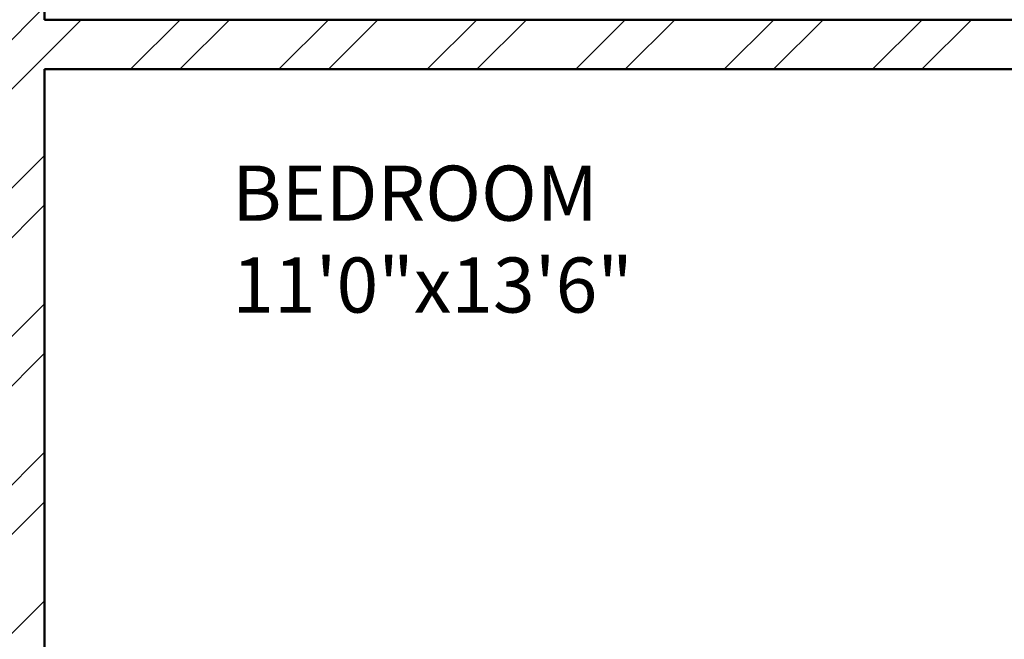
# Model space of a CAD drawing. Units: inches. Extents: x 963 to 2075, y 289 to 2657.
# Tile 43 of 98: x 1511 to 1600, y 1658 to 1714. Entities that reach past the tile are written whole.
import ezdxf

# ---------------------------------------------------------------- set-up
doc = ezdxf.new("R2010")
doc.units = ezdxf.units.IN
for name, color, linetype, lineweight in [('A-AREA-IDEN', 7, 'Continuous', 18), ('A-WALL', 7, 'Continuous', 50), ('A-WALL-PATT', 8, 'Continuous', 13)]:
    doc.layers.add(name, color=color, linetype=linetype, lineweight=lineweight)
doc.styles.get("Standard").update_dxf_attribs({"font": 'arial.ttf'})

msp = doc.modelspace()

# ---------------------------------------------------------------- hatches: boundary and pattern name
at = {"layer": 'A-WALL-PATT'}
h = msp.add_hatch(dxfattribs=at)
h.set_pattern_fill('ANSI32', color=256)
h.paths.add_polyline_path([(1296.922, 2558.318), (1203.922, 2558.318), (1203.922, 2493.818), (1191.533, 2493.818), (1191.533, 2489.318), (1211.063, 2489.318), (1211.063, 2492.02), (1211.063, 2493.818), (1208.422, 2493.818), (1208.422, 2553.818), (1292.422, 2553.818), (1292.422, 2538.863), (1296.922, 2538.863)])
h.paths.add_polyline_path([(1442.422, 2558.318), (1349.422, 2558.318), (1349.422, 2538.943), (1353.922, 2538.943), (1353.922, 2553.818), (1437.922, 2553.818), (1437.922, 2493.818), (1434.542, 2493.818), (1434.542, 2489.318), (1448.311, 2489.318), (1448.311, 2491.568), (1448.311, 2493.818), (1442.422, 2493.818)])
h.paths.add_polyline_path([(1415.554, 2491.568), (1415.554, 2493.818), (1340.941, 2493.818), (1340.941, 2489.318), (1371.922, 2489.318), (1371.922, 2378.318), (1367.596, 2378.318), (1367.596, 2373.818), (1371.922, 2373.818), (1371.922, 2355.185), (1376.422, 2355.185), (1376.422, 2489.318), (1415.554, 2489.318)])
h.paths.add_polyline_path([(1304.941, 2491.568), (1304.941, 2493.818), (1296.922, 2493.818), (1296.922, 2514.863), (1292.422, 2514.863), (1292.422, 2493.818), (1232.808, 2493.818), (1232.808, 2489.318), (1256.422, 2489.318), (1256.422, 2327.318), (1253.714, 2327.318), (1253.714, 2322.818), (1328.422, 2322.818), (1328.422, 2331.147), (1323.922, 2331.147), (1323.922, 2327.318), (1260.922, 2327.318), (1260.922, 2373.818), (1323.922, 2373.818), (1323.922, 2357.812), (1328.422, 2357.812), (1328.422, 2373.818), (1346.007, 2373.818), (1346.007, 2376.068), (1346.007, 2378.318), (1260.922, 2378.318), (1260.922, 2489.318), (1304.941, 2489.318)])
h.paths.add_polyline_path([(1226.654, 2327.318), (1124.422, 2327.318), (1124.422, 2347.447), (1119.922, 2347.447), (1119.922, 2322.818), (1163.422, 2322.818), (1163.422, 2305.435), (1165.672, 2305.435), (1167.922, 2305.435), (1167.922, 2322.818), (1226.654, 2322.818), (1226.654, 2325.068)])
h.paths.add_polyline_path([(1095.922, 2489.318), (1124.422, 2489.318), (1131.533, 2489.318), (1131.533, 2491.568), (1131.533, 2493.818), (1119.922, 2493.818), (1091.422, 2493.818), (1091.422, 2417.318), (1095.922, 2417.318), (1119.922, 2417.318), (1119.922, 2407.447), (1124.422, 2407.447), (1124.422, 2421.818), (1095.922, 2421.818)])
h.paths.add_polyline_path([(1512.922, 2558.318), (1508.422, 2558.318), (1508.422, 2493.818), (1503.401, 2493.818), (1503.401, 2489.318), (1508.422, 2489.318), (1508.422, 2327.318), (1376.422, 2327.318), (1376.422, 2330.273), (1371.922, 2330.273), (1371.922, 2298.744), (1376.422, 2298.744), (1376.422, 2322.818), (1508.422, 2322.818), (1508.422, 2165.318), (1504.255, 2165.318), (1504.255, 2160.818), (1508.422, 2160.818), (1508.422, 2108.318), (1512.922, 2108.318), (1512.922, 2160.818), (1516.182, 2160.818), (1516.182, 2163.068), (1516.182, 2165.318), (1512.922, 2165.318), (1512.922, 2322.818), (1644.922, 2322.818), (1644.922, 2298.744), (1649.422, 2298.744), (1649.422, 2322.818), (1649.422, 2330.944), (1647.172, 2330.944), (1644.922, 2330.944), (1644.922, 2327.318), (1512.922, 2327.318), (1512.922, 2489.318), (1516.759, 2489.318), (1516.759, 2491.568), (1516.759, 2493.818), (1512.922, 2493.818)])
h.paths.add_polyline_path([(1671.922, 2558.318), (1578.922, 2558.318), (1578.922, 2493.818), (1573.526, 2493.818), (1573.526, 2489.318), (1586.537, 2489.318), (1586.537, 2491.568), (1586.537, 2493.818), (1583.422, 2493.818), (1583.422, 2553.818), (1667.422, 2553.818), (1667.422, 2541.109), (1671.922, 2541.109)])
h.paths.add_polyline_path([(1681.257, 2493.818), (1671.922, 2493.818), (1671.922, 2517.109), (1667.422, 2517.109), (1667.422, 2493.818), (1610.218, 2493.818), (1610.218, 2489.318), (1644.922, 2489.318), (1644.922, 2357.865), (1649.422, 2357.865), (1649.422, 2373.818), (1652.203, 2373.818), (1652.203, 2375.827), (1652.203, 2378.318), (1649.422, 2378.318), (1649.422, 2489.318), (1681.257, 2489.318), (1681.257, 2491.568)])
h.paths.add_polyline_path([(1821.922, 2558.318), (1728.922, 2558.318), (1728.922, 2541), (1733.422, 2541), (1733.422, 2553.818), (1817.422, 2553.818), (1817.422, 2493.818), (1813.507, 2493.818), (1813.507, 2489.318), (1830.078, 2489.318), (1830.078, 2491.568), (1830.078, 2493.818), (1821.922, 2493.818)])
h.paths.add_polyline_path([(1794.244, 2493.818), (1717.257, 2493.818), (1717.257, 2489.318), (1760.422, 2489.318), (1760.422, 2378.318), (1674.401, 2378.318), (1674.401, 2373.818), (1692.922, 2373.818), (1692.922, 2356.954), (1697.422, 2356.954), (1697.422, 2373.818), (1760.422, 2373.818), (1760.422, 2327.318), (1697.422, 2327.318), (1697.422, 2333.341), (1692.922, 2333.341), (1692.922, 2322.818), (1768.037, 2322.818), (1768.037, 2325.068), (1768.037, 2327.318), (1764.922, 2327.318), (1764.922, 2489.318), (1794.244, 2489.318)])
h.paths.add_polyline_path([(1733.422, 2517), (1728.922, 2517), (1728.922, 2493.818), (1733.422, 2493.818)], flags=17)
h.paths.add_polyline_path([(1929.922, 2493.818), (1890.078, 2493.818), (1890.078, 2489.318), (1896.922, 2489.318), (1925.422, 2489.318), (1925.422, 2421.818), (1896.922, 2421.818), (1896.922, 2408.318), (1901.422, 2408.318), (1901.422, 2417.318), (1925.422, 2417.318), (1929.922, 2417.318)])
h.paths.add_polyline_path([(1901.422, 2348.318), (1896.922, 2348.318), (1896.922, 2327.318), (1800.423, 2327.318), (1800.423, 2322.818), (1853.422, 2322.818), (1853.422, 2309.453), (1857.922, 2309.453), (1857.922, 2322.818), (1901.422, 2322.818)])
h.paths.add_polyline_path([(1857.922, 2249.453), (1853.422, 2249.453), (1853.422, 2214.818), (1686.309, 2214.818), (1686.309, 2210.318), (1853.422, 2210.318), (1853.422, 2202.134), (1857.922, 2202.134), (1857.922, 2210.318)])
h.paths.add_polyline_path([(1857.922, 2142.134), (1853.422, 2142.134), (1853.422, 2115.422), (1841.422, 2115.422), (1841.422, 2088.531), (1841.422, 2046.949), (1845.922, 2046.949), (1845.922, 2110.922), (1905.922, 2110.922), (1905.922, 2092.517), (1910.422, 2092.517), (1910.422, 2115.422), (1857.922, 2115.422)])
h.paths.add_polyline_path([(1532.436, 1482.342), (1573.456, 1482.342), (1573.456, 1501), (1532.436, 1501)], flags=9)
h.paths.add_polyline_path([(1438.658, 1486.302), (1479.678, 1486.302), (1479.678, 1504.96), (1438.658, 1504.96)], flags=9)
h.paths.add_polyline_path([(1411.215, 1365.308), (1659.139, 1365.308), (1659.139, 1402.401), (1411.215, 1402.401)], flags=9)
h.paths.add_polyline_path([(1185.671, 2296.298), (1248.16, 2296.298), (1248.16, 2314.955), (1185.671, 2314.955)], flags=9)
h.paths.add_polyline_path([(1177.31, 2187.35), (1216.15, 2187.35), (1216.15, 2206.007), (1177.31, 2206.007)], flags=9)
h.paths.add_polyline_path([(1295.101, 1602.083), (1328.26, 1602.083), (1328.26, 1620.741), (1295.101, 1620.741)], flags=9)
h.paths.add_polyline_path([(1525.126, 2005.99), (1558.39, 2005.99), (1558.39, 2024.648), (1525.126, 2024.648)], flags=9)
h.paths.add_polyline_path([(1459.606, 1977.125), (1472.195, 1977.125), (1472.195, 1987.429), (1459.606, 1987.429)], flags=9)
h.paths.add_polyline_path([(1467.815, 2053.676), (1480.018, 2053.676), (1480.018, 2063.979), (1467.815, 2063.979)], flags=9)
h.paths.add_polyline_path([(1555.184, 2119.02), (1584.563, 2119.02), (1584.563, 2137.678), (1555.184, 2137.678)], flags=25)
h.paths.add_polyline_path([(1405.389, 2115.291), (1444.478, 2115.291), (1444.478, 2133.948), (1405.389, 2133.948)], flags=25)
h.paths.add_polyline_path([(1698.482, 2004.259), (1727.695, 2004.259), (1727.695, 2022.916), (1698.482, 2022.916)], flags=9)
h.paths.add_polyline_path([(1612.158, 1972.855), (1629.016, 1972.855), (1629.016, 1983.159), (1612.158, 1983.159)], flags=9)
h.paths.add_polyline_path([(1608.289, 2060.036), (1625.147, 2060.036), (1625.147, 2070.34), (1608.289, 2070.34)], flags=9)
h.paths.add_polyline_path([(1527.954, 1684.402), (1566.795, 1684.402), (1566.795, 1703.06), (1527.954, 1703.06)], flags=9)
h.paths.add_polyline_path([(1422.792, 1683.59), (1461.633, 1683.59), (1461.633, 1702.247), (1422.792, 1702.247)], flags=9)
h.paths.add_polyline_path([(1531.262, 1732.459), (1574.015, 1732.459), (1574.015, 1751.116), (1531.262, 1751.116)], flags=9)
h.paths.add_polyline_path([(1402.872, 1732.845), (1439.799, 1732.845), (1439.799, 1751.502), (1402.872, 1751.502)], flags=9)
h.paths.add_polyline_path([(1243.122, 1923.132), (1281.962, 1923.132), (1281.962, 1941.79), (1243.122, 1941.79)], flags=9)
h.paths.add_polyline_path([(1181.752, 1792.268), (1244.241, 1792.268), (1244.241, 1810.926), (1181.752, 1810.926)], flags=9)
h.paths.add_polyline_path([(1265.822, 1670.3), (1316.071, 1670.3), (1316.071, 1688.957), (1265.822, 1688.957)], flags=9)
h.paths.add_polyline_path([(1140.263, 1676.054), (1179.104, 1676.054), (1179.104, 1694.711), (1140.263, 1694.711)], flags=9)
h.paths.add_polyline_path([(1107.49, 1490.889), (1143.374, 1490.889), (1143.374, 1509.546), (1107.49, 1509.546)], flags=9)
h.paths.add_polyline_path([(1217.584, 1483.899), (1246.741, 1483.899), (1246.741, 1502.556), (1217.584, 1502.556)], flags=9)
h.paths.add_polyline_path([(1389.21, 1486.919), (1418.367, 1486.919), (1418.367, 1505.576), (1389.21, 1505.576)], flags=9)
h.paths.add_polyline_path([(1672.208, 1602.083), (1705.366, 1602.083), (1705.366, 1620.741), (1672.208, 1620.741)], flags=9)
h.paths.add_polyline_path([(1752.082, 1522.638), (1781.24, 1522.638), (1781.24, 1541.295), (1752.082, 1541.295)], flags=9)
h.paths.add_polyline_path([(1848.275, 1491.26), (1884.158, 1491.26), (1884.158, 1509.918), (1848.275, 1509.918)], flags=9)
h.paths.add_polyline_path([(1822.47, 1685.62), (1861.31, 1685.62), (1861.31, 1704.278), (1822.47, 1704.278)], flags=9)
h.paths.add_polyline_path([(1713.195, 1672.232), (1763.444, 1672.232), (1763.444, 1690.889), (1713.195, 1690.889)], flags=9)
h.paths.add_polyline_path([(1736.619, 1790.578), (1799.109, 1790.578), (1799.109, 1809.235), (1736.619, 1809.235)], flags=9)
h.paths.add_polyline_path([(1691.491, 1916.355), (1730.332, 1916.355), (1730.332, 1935.013), (1691.491, 1935.013)], flags=9)
h.paths.add_polyline_path([(1764.872, 1973.922), (1794.306, 1973.922), (1794.306, 1992.58), (1764.872, 1992.58)], flags=9)
h.paths.add_polyline_path([(1767.854, 2034.017), (1797.288, 2034.017), (1797.288, 2052.674), (1767.854, 2052.674)], flags=9)
h.paths.add_polyline_path([(1851.593, 2060.331), (1880.751, 2060.331), (1880.751, 2078.989), (1851.593, 2078.989)], flags=25)
h.paths.add_polyline_path([(1688.491, 2086.874), (1727.332, 2086.874), (1727.332, 2105.531), (1688.491, 2105.531)], flags=9)
h.paths.add_polyline_path([(1537.743, 2293.581), (1580.495, 2293.581), (1580.495, 2312.239), (1537.743, 2312.239)], flags=25)
h.paths.add_polyline_path([(1425.587, 2296.109), (1468.34, 2296.109), (1468.34, 2314.766), (1425.587, 2314.766)], flags=25)
h.paths.add_polyline_path([(1278.518, 2004.184), (1307.72, 2004.184), (1307.72, 2022.841), (1278.518, 2022.841)], flags=9)
h.paths.add_polyline_path([(1193.282, 1973.635), (1222.715, 1973.635), (1222.715, 1992.292), (1193.282, 1992.292)], flags=9)
h.paths.add_polyline_path([(1192.411, 2040.577), (1221.845, 2040.577), (1221.845, 2059.234), (1192.411, 2059.234)], flags=9)
h.paths.add_polyline_path([(1130.603, 1951.393), (1159.76, 1951.393), (1159.76, 1970.05), (1130.603, 1970.05)], flags=9)
h.paths.add_polyline_path([(1132.827, 2052.494), (1161.984, 2052.494), (1161.984, 2071.151), (1132.827, 2071.151)], flags=9)
h.paths.add_polyline_path([(1265.128, 2334.619), (1315.377, 2334.619), (1315.377, 2353.277), (1265.128, 2353.277)], flags=25)
h.paths.add_polyline_path([(1136.741, 2330.785), (1175.582, 2330.785), (1175.582, 2349.443), (1136.741, 2349.443)], flags=9)
h.paths.add_polyline_path([(1287.422, 2417.204), (1320.58, 2417.204), (1320.58, 2435.861), (1287.422, 2435.861)], flags=25)
h.paths.add_polyline_path([(1430.988, 2329.159), (1469.828, 2329.159), (1469.828, 2347.816), (1430.988, 2347.816)], flags=25)
h.paths.add_polyline_path([(1525.424, 2329.213), (1564.264, 2329.213), (1564.264, 2347.87), (1525.424, 2347.87)], flags=25)
h.paths.add_polyline_path([(1684.525, 2382.799), (1717.683, 2382.799), (1717.683, 2401.457), (1684.525, 2401.457)], flags=25)
h.paths.add_polyline_path([(1704.805, 2340.293), (1755.054, 2340.293), (1755.054, 2358.95), (1704.805, 2358.95)], flags=25)
h.paths.add_polyline_path([(1694.113, 2287.757), (1756.602, 2287.757), (1756.602, 2306.414), (1694.113, 2306.414)], flags=9)
h.paths.add_polyline_path([(1815.778, 2329.861), (1854.618, 2329.861), (1854.618, 2348.518), (1815.778, 2348.518)], flags=9)
h.paths.add_polyline_path([(1842.873, 2514.256), (1878.756, 2514.256), (1878.756, 2532.914), (1842.873, 2532.914)], flags=9)
h.paths.add_polyline_path([(1769.513, 2531.447), (1798.671, 2531.447), (1798.671, 2550.104), (1769.513, 2550.104)], flags=25)
h.paths.add_polyline_path([(1594.772, 2518.468), (1623.93, 2518.468), (1623.93, 2537.125), (1594.772, 2537.125)], flags=25)
h.paths.add_polyline_path([(1520.723, 2516.185), (1556.606, 2516.185), (1556.606, 2534.842), (1520.723, 2534.842)], flags=25)
h.paths.add_polyline_path([(1464.456, 2516.694), (1500.34, 2516.694), (1500.34, 2535.351), (1464.456, 2535.351)], flags=25)
h.paths.add_polyline_path([(1365.696, 2528.97), (1394.854, 2528.97), (1394.854, 2547.627), (1365.696, 2547.627)], flags=25)
h.paths.add_polyline_path([(1222.838, 2516.231), (1251.995, 2516.231), (1251.995, 2534.889), (1222.838, 2534.889)], flags=25)
h.paths.add_polyline_path([(1104.545, 2509.6), (1140.429, 2509.6), (1140.429, 2528.257), (1104.545, 2528.257)], flags=9)
h = msp.add_hatch(dxfattribs=at)
h.set_pattern_fill('ANSI32', color=256)
h.paths.add_polyline_path([(1335.968, 2212.568), (1335.968, 2214.818), (1167.922, 2214.818), (1167.922, 2245.435), (1163.422, 2245.435), (1163.422, 2210.318), (1163.422, 2194.812), (1167.922, 2194.812), (1167.922, 2210.318), (1335.968, 2210.318)])
h.paths.add_polyline_path([(1532.436, 1482.342), (1573.456, 1482.342), (1573.456, 1501), (1532.436, 1501)], flags=9)
h.paths.add_polyline_path([(1438.658, 1486.302), (1479.678, 1486.302), (1479.678, 1504.96), (1438.658, 1504.96)], flags=9)
h.paths.add_polyline_path([(1411.215, 1365.308), (1659.139, 1365.308), (1659.139, 1402.401), (1411.215, 1402.401)], flags=9)
h.paths.add_polyline_path([(1185.671, 2296.298), (1248.16, 2296.298), (1248.16, 2314.955), (1185.671, 2314.955)], flags=9)
h.paths.add_polyline_path([(1177.31, 2187.35), (1216.15, 2187.35), (1216.15, 2206.007), (1177.31, 2206.007)], flags=9)
h.paths.add_polyline_path([(1295.101, 1602.083), (1328.26, 1602.083), (1328.26, 1620.741), (1295.101, 1620.741)], flags=9)
h.paths.add_polyline_path([(1525.126, 2005.99), (1558.39, 2005.99), (1558.39, 2024.648), (1525.126, 2024.648)], flags=9)
h.paths.add_polyline_path([(1459.606, 1977.125), (1472.195, 1977.125), (1472.195, 1987.429), (1459.606, 1987.429)], flags=9)
h.paths.add_polyline_path([(1467.815, 2053.676), (1480.018, 2053.676), (1480.018, 2063.979), (1467.815, 2063.979)], flags=9)
h.paths.add_polyline_path([(1555.184, 2119.02), (1584.563, 2119.02), (1584.563, 2137.678), (1555.184, 2137.678)], flags=9)
h.paths.add_polyline_path([(1405.389, 2115.291), (1444.478, 2115.291), (1444.478, 2133.948), (1405.389, 2133.948)], flags=9)
h.paths.add_polyline_path([(1698.482, 2004.259), (1727.695, 2004.259), (1727.695, 2022.916), (1698.482, 2022.916)], flags=9)
h.paths.add_polyline_path([(1612.158, 1972.855), (1629.016, 1972.855), (1629.016, 1983.159), (1612.158, 1983.159)], flags=9)
h.paths.add_polyline_path([(1608.289, 2060.036), (1625.147, 2060.036), (1625.147, 2070.34), (1608.289, 2070.34)], flags=9)
h.paths.add_polyline_path([(1527.954, 1684.402), (1566.795, 1684.402), (1566.795, 1703.06), (1527.954, 1703.06)], flags=9)
h.paths.add_polyline_path([(1422.792, 1683.59), (1461.633, 1683.59), (1461.633, 1702.247), (1422.792, 1702.247)], flags=9)
h.paths.add_polyline_path([(1531.262, 1732.459), (1574.015, 1732.459), (1574.015, 1751.116), (1531.262, 1751.116)], flags=9)
h.paths.add_polyline_path([(1402.872, 1732.845), (1439.799, 1732.845), (1439.799, 1751.502), (1402.872, 1751.502)], flags=9)
h.paths.add_polyline_path([(1243.122, 1923.132), (1281.962, 1923.132), (1281.962, 1941.79), (1243.122, 1941.79)], flags=9)
h.paths.add_polyline_path([(1181.752, 1792.268), (1244.241, 1792.268), (1244.241, 1810.926), (1181.752, 1810.926)], flags=9)
h.paths.add_polyline_path([(1265.822, 1670.3), (1316.071, 1670.3), (1316.071, 1688.957), (1265.822, 1688.957)], flags=9)
h.paths.add_polyline_path([(1140.263, 1676.054), (1179.104, 1676.054), (1179.104, 1694.711), (1140.263, 1694.711)], flags=9)
h.paths.add_polyline_path([(1107.49, 1490.889), (1143.374, 1490.889), (1143.374, 1509.546), (1107.49, 1509.546)], flags=9)
h.paths.add_polyline_path([(1217.584, 1483.899), (1246.741, 1483.899), (1246.741, 1502.556), (1217.584, 1502.556)], flags=9)
h.paths.add_polyline_path([(1389.21, 1486.919), (1418.367, 1486.919), (1418.367, 1505.576), (1389.21, 1505.576)], flags=9)
h.paths.add_polyline_path([(1672.208, 1602.083), (1705.366, 1602.083), (1705.366, 1620.741), (1672.208, 1620.741)], flags=9)
h.paths.add_polyline_path([(1752.082, 1522.638), (1781.24, 1522.638), (1781.24, 1541.295), (1752.082, 1541.295)], flags=9)
h.paths.add_polyline_path([(1848.275, 1491.26), (1884.158, 1491.26), (1884.158, 1509.918), (1848.275, 1509.918)], flags=9)
h.paths.add_polyline_path([(1822.47, 1685.62), (1861.31, 1685.62), (1861.31, 1704.278), (1822.47, 1704.278)], flags=9)
h.paths.add_polyline_path([(1713.195, 1672.232), (1763.444, 1672.232), (1763.444, 1690.889), (1713.195, 1690.889)], flags=9)
h.paths.add_polyline_path([(1736.619, 1790.578), (1799.109, 1790.578), (1799.109, 1809.235), (1736.619, 1809.235)], flags=9)
h.paths.add_polyline_path([(1691.491, 1916.355), (1730.332, 1916.355), (1730.332, 1935.013), (1691.491, 1935.013)], flags=9)
h.paths.add_polyline_path([(1764.872, 1973.922), (1794.306, 1973.922), (1794.306, 1992.58), (1764.872, 1992.58)], flags=9)
h.paths.add_polyline_path([(1767.854, 2034.017), (1797.288, 2034.017), (1797.288, 2052.674), (1767.854, 2052.674)], flags=9)
h.paths.add_polyline_path([(1851.593, 2060.331), (1880.751, 2060.331), (1880.751, 2078.989), (1851.593, 2078.989)], flags=9)
h.paths.add_polyline_path([(1688.491, 2086.874), (1727.332, 2086.874), (1727.332, 2105.531), (1688.491, 2105.531)], flags=9)
h.paths.add_polyline_path([(1537.743, 2293.581), (1580.495, 2293.581), (1580.495, 2312.239), (1537.743, 2312.239)], flags=9)
h.paths.add_polyline_path([(1425.587, 2296.109), (1468.34, 2296.109), (1468.34, 2314.766), (1425.587, 2314.766)], flags=9)
h.paths.add_polyline_path([(1278.518, 2004.184), (1307.72, 2004.184), (1307.72, 2022.841), (1278.518, 2022.841)], flags=9)
h.paths.add_polyline_path([(1193.282, 1973.635), (1222.715, 1973.635), (1222.715, 1992.292), (1193.282, 1992.292)], flags=9)
h.paths.add_polyline_path([(1192.411, 2040.577), (1221.845, 2040.577), (1221.845, 2059.234), (1192.411, 2059.234)], flags=9)
h.paths.add_polyline_path([(1130.603, 1951.393), (1159.76, 1951.393), (1159.76, 1970.05), (1130.603, 1970.05)], flags=9)
h.paths.add_polyline_path([(1132.827, 2052.494), (1161.984, 2052.494), (1161.984, 2071.151), (1132.827, 2071.151)], flags=9)
h.paths.add_polyline_path([(1265.128, 2334.619), (1315.377, 2334.619), (1315.377, 2353.277), (1265.128, 2353.277)], flags=9)
h.paths.add_polyline_path([(1136.741, 2330.785), (1175.582, 2330.785), (1175.582, 2349.443), (1136.741, 2349.443)], flags=9)
h.paths.add_polyline_path([(1287.422, 2417.204), (1320.58, 2417.204), (1320.58, 2435.861), (1287.422, 2435.861)], flags=9)
h.paths.add_polyline_path([(1430.988, 2329.159), (1469.828, 2329.159), (1469.828, 2347.816), (1430.988, 2347.816)], flags=9)
h.paths.add_polyline_path([(1525.424, 2329.213), (1564.264, 2329.213), (1564.264, 2347.87), (1525.424, 2347.87)], flags=9)
h.paths.add_polyline_path([(1684.525, 2382.799), (1717.683, 2382.799), (1717.683, 2401.457), (1684.525, 2401.457)], flags=9)
h.paths.add_polyline_path([(1704.805, 2340.293), (1755.054, 2340.293), (1755.054, 2358.95), (1704.805, 2358.95)], flags=9)
h.paths.add_polyline_path([(1694.113, 2287.757), (1756.602, 2287.757), (1756.602, 2306.414), (1694.113, 2306.414)], flags=9)
h.paths.add_polyline_path([(1815.778, 2329.861), (1854.618, 2329.861), (1854.618, 2348.518), (1815.778, 2348.518)], flags=9)
h.paths.add_polyline_path([(1842.873, 2514.256), (1878.756, 2514.256), (1878.756, 2532.914), (1842.873, 2532.914)], flags=9)
h.paths.add_polyline_path([(1769.513, 2531.447), (1798.671, 2531.447), (1798.671, 2550.104), (1769.513, 2550.104)], flags=9)
h.paths.add_polyline_path([(1594.772, 2518.468), (1623.93, 2518.468), (1623.93, 2537.125), (1594.772, 2537.125)], flags=9)
h.paths.add_polyline_path([(1520.723, 2516.185), (1556.606, 2516.185), (1556.606, 2534.842), (1520.723, 2534.842)], flags=9)
h.paths.add_polyline_path([(1464.456, 2516.694), (1500.34, 2516.694), (1500.34, 2535.351), (1464.456, 2535.351)], flags=9)
h.paths.add_polyline_path([(1365.696, 2528.97), (1394.854, 2528.97), (1394.854, 2547.627), (1365.696, 2547.627)], flags=9)
h.paths.add_polyline_path([(1222.838, 2516.231), (1251.995, 2516.231), (1251.995, 2534.889), (1222.838, 2534.889)], flags=9)
h.paths.add_polyline_path([(1104.545, 2509.6), (1140.429, 2509.6), (1140.429, 2528.257), (1104.545, 2528.257)], flags=9)
h = msp.add_hatch(dxfattribs=at)
h.set_pattern_fill('ANSI32', color=256)
h.paths.add_polyline_path([(1473.609, 2163.068), (1473.609, 2165.318), (1376.422, 2165.318), (1376.422, 2227.983), (1371.922, 2227.983), (1371.922, 2214.818), (1368.405, 2214.818), (1368.405, 2210.318), (1371.922, 2210.318), (1371.922, 2160.818), (1395.922, 2160.818), (1395.922, 2090.318), (1217.345, 2090.318), (1217.345, 2085.818), (1395.922, 2085.818), (1458.922, 2085.818), (1458.922, 2108.318), (1454.422, 2108.318), (1454.422, 2090.318), (1400.422, 2090.318), (1400.422, 2160.818), (1473.609, 2160.818)])
h.paths.add_polyline_path([(1649.422, 2210.318), (1653.225, 2210.318), (1653.225, 2214.818), (1649.422, 2214.818), (1649.422, 2227.983), (1644.922, 2227.983), (1644.922, 2165.318), (1550.099, 2165.318), (1550.099, 2160.818), (1620.922, 2160.818), (1620.922, 2112.818), (1555.446, 2112.818), (1555.446, 2108.318), (1584.327, 2108.318), (1584.327, 2084.916), (1588.827, 2084.916), (1588.827, 2108.318), (1625.422, 2108.318), (1667.951, 2108.318), (1667.951, 2022.667), (1588.827, 2022.667), (1588.827, 2047.408), (1584.327, 2047.408), (1584.327, 1996.003), (1588.827, 1996.003), (1588.827, 2018.318), (1667.951, 2018.167), (1667.951, 1928.318), (1625.422, 1928.318), (1625.422, 1923.818), (1672.451, 1923.818), (1672.451, 1928.318), (1672.451, 1946.663), (1785.446, 1946.663), (1785.446, 1951.163), (1743.034, 1951.163), (1743.034, 2017.922), (1841.422, 2017.922), (1841.422, 2014.775), (1845.922, 2014.775), (1845.922, 2017.922), (1905.922, 2017.922), (1905.922, 1987.511), (1910.422, 1987.511), (1910.422, 2022.422), (1910.422, 2068.517), (1905.922, 2068.517), (1905.922, 2022.422), (1845.922, 2022.422), (1845.922, 2025.851), (1843.672, 2025.851), (1841.422, 2025.851), (1841.422, 2022.422), (1743.034, 2022.422), (1743.034, 2084.031), (1768.451, 2084.031), (1785.446, 2084.031), (1785.446, 2088.531), (1672.451, 2088.531), (1672.451, 2112.818), (1667.951, 2112.818), (1625.422, 2112.818), (1625.422, 2160.818), (1649.422, 2160.818)])
h.paths.add_polyline_path([(1672.451, 2084.031), (1738.534, 2084.031), (1738.534, 1951.163), (1672.451, 1951.163)], flags=16)
h.paths.add_polyline_path([(1672.451, 2084.031), (1738.534, 2084.031), (1705.492, 2017.597)], flags=0)
h.paths.add_polyline_path([(1262.766, 2085.818), (1258.266, 2085.818), (1258.266, 2023.278), (1184.422, 2023.278), (1184.422, 2018.778), (1258.266, 2018.778), (1258.266, 1950.818), (1262.766, 1950.818)])
h.paths.add_polyline_path([(1312.266, 2085.818), (1307.766, 2085.818), (1307.766, 1950.818), (1312.266, 1950.818)])
h.paths.add_polyline_path([(1458.922, 1950.818), (1395.922, 1950.818), (1216.568, 1950.818), (1216.568, 1946.318), (1346.422, 1946.318), (1395.922, 1946.318), (1395.922, 1875.818), (1371.922, 1875.818), (1371.922, 1826.318), (1368.931, 1826.318), (1368.931, 1821.818), (1371.922, 1821.818), (1371.922, 1813.622), (1376.422, 1813.622), (1376.422, 1871.318), (1474.504, 1871.318), (1474.504, 1873.568), (1474.504, 1875.818), (1400.422, 1875.818), (1400.422, 1946.318), (1454.422, 1946.318), (1454.422, 1928.318), (1458.922, 1928.318)])
h.paths.add_polyline_path([(1184.422, 2120.778), (1167.922, 2120.778), (1167.922, 2134.812), (1165.672, 2134.812), (1163.422, 2134.812), (1163.422, 2120.778), (1119.922, 2120.778), (1119.922, 2098.095), (1124.422, 2098.095), (1124.422, 2116.278), (1167.922, 2116.278), (1179.922, 2116.278), (1179.922, 2045.916), (1184.422, 2045.916), (1184.422, 2090.318), (1184.422, 2116.278)])
h.paths.add_polyline_path([(1124.422, 2018.778), (1179.922, 2018.778), (1179.922, 2016.294), (1184.422, 2016.294), (1184.422, 2023.278), (1184.422, 2026.588), (1182.172, 2026.588), (1179.922, 2026.588), (1179.922, 2023.278), (1124.422, 2023.278), (1124.422, 2074.095), (1119.922, 2074.095), (1119.922, 2018.778), (1119.922, 1979.633), (1124.422, 1979.633)])
h.paths.add_polyline_path([(1184.422, 1925.778), (1184.422, 1946.318), (1184.422, 1996.073), (1182.172, 1996.073), (1179.922, 1996.073), (1179.922, 1925.778), (1124.422, 1925.778), (1124.422, 1955.633), (1119.922, 1955.502), (1119.922, 1921.278), (1158.922, 1921.278), (1158.922, 1909.983), (1163.422, 1909.983), (1163.422, 1921.278), (1184.422, 1921.278)])
h.paths.add_polyline_path([(1341.449, 1826.318), (1163.422, 1826.318), (1163.422, 1849.983), (1158.922, 1849.983), (1158.922, 1821.818), (1158.922, 1804.033), (1163.422, 1804.033), (1163.422, 1821.818), (1341.449, 1821.818)])
h.paths.add_polyline_path([(1222.981, 1713.818), (1163.422, 1713.818), (1163.422, 1744.033), (1161.172, 1744.033), (1158.922, 1744.033), (1158.922, 1713.818), (1119.922, 1713.818), (1119.922, 1694.65), (1124.422, 1694.65), (1124.422, 1709.318), (1158.922, 1709.318), (1222.981, 1709.318)])
h.paths.add_polyline_path([(1328.422, 1713.818), (1252.042, 1713.818), (1252.042, 1711.568), (1252.042, 1709.318), (1256.422, 1709.318), (1256.422, 1547.318), (1232.937, 1547.318), (1232.937, 1545.068), (1232.937, 1542.818), (1292.422, 1542.818), (1292.422, 1527.634), (1296.922, 1527.634), (1296.922, 1542.818), (1299.464, 1542.818), (1299.464, 1547.318), (1260.922, 1547.318), (1260.922, 1658.318), (1343.661, 1658.318), (1343.661, 1660.568), (1343.661, 1662.818), (1328.422, 1662.818), (1328.422, 1676.589), (1327.402, 1676.589), (1323.922, 1676.589), (1323.922, 1662.818), (1260.922, 1662.818), (1260.922, 1709.318), (1323.922, 1709.318), (1323.922, 1699.851), (1328.422, 1699.851)])
h.paths.add_polyline_path([(1649.422, 1875.818), (1625.422, 1875.818), (1625.422, 1928.318), (1620.922, 1928.318), (1588.827, 1928.318), (1588.827, 1950.59), (1584.327, 1950.59), (1584.327, 1928.318), (1555.446, 1928.318), (1555.446, 1923.818), (1620.922, 1923.818), (1620.922, 1875.818), (1548.952, 1875.818), (1548.952, 1873.568), (1548.952, 1871.318), (1644.922, 1871.318), (1644.922, 1813.622), (1649.422, 1813.622), (1649.422, 1821.818), (1652.045, 1821.818), (1652.045, 1824.068), (1652.045, 1826.318), (1649.422, 1826.318)])
h.paths.add_polyline_path([(1512.922, 1871.318), (1516.476, 1871.318), (1516.476, 1875.818), (1512.922, 1875.818), (1512.922, 1923.818), (1512.922, 1928.318), (1512.922, 1930.827), (1508.422, 1930.827), (1508.422, 1875.818), (1504.411, 1875.818), (1504.411, 1871.318), (1508.422, 1871.318), (1508.422, 1713.818), (1376.422, 1713.818), (1376.422, 1743.325), (1371.922, 1743.325), (1371.922, 1709.318), (1371.922, 1706.01), (1376.422, 1706.01), (1376.422, 1709.318), (1508.422, 1709.318), (1508.422, 1547.318), (1501.871, 1547.318), (1501.871, 1542.818), (1508.422, 1542.818), (1508.422, 1482.818), (1508.422, 1436.318), (1512.922, 1436.318), (1512.922, 1542.818), (1519.318, 1542.818), (1519.318, 1545.068), (1519.318, 1547.318), (1512.922, 1547.318), (1512.922, 1709.318), (1644.922, 1709.318), (1644.922, 1707.548), (1649.422, 1707.548), (1649.422, 1709.318), (1649.422, 1743.325), (1644.922, 1743.325), (1644.922, 1713.818), (1512.922, 1713.818)])
h.paths.add_polyline_path([(1129.884, 1545.068), (1129.884, 1547.318), (1124.422, 1547.318), (1095.922, 1547.318), (1095.922, 1614.818), (1124.422, 1614.818), (1124.422, 1619.318), (1095.922, 1619.318), (1091.422, 1619.318), (1091.422, 1542.818), (1095.922, 1542.818), (1119.922, 1542.818), (1129.884, 1542.818)])
h.paths.add_polyline_path([(1208.422, 1542.818), (1211.74, 1542.818), (1211.74, 1547.318), (1198.851, 1547.318), (1198.851, 1542.818), (1203.922, 1542.818), (1203.922, 1478.318), (1208.422, 1478.318), (1296.922, 1478.318), (1296.922, 1503.634), (1292.422, 1503.634), (1292.422, 1482.818), (1208.422, 1482.818)])
h.paths.add_polyline_path([(1430.422, 1542.818), (1435.699, 1542.818), (1435.699, 1545.068), (1435.699, 1547.318), (1422.658, 1547.318), (1422.658, 1545.068), (1422.658, 1542.818), (1425.922, 1542.818), (1425.922, 1482.857), (1341.922, 1482.857), (1341.922, 1502.732), (1337.422, 1502.732), (1337.422, 1478.357), (1425.922, 1478.357), (1425.922, 1440.818), (1425.922, 1436.318), (1430.422, 1436.318)])
h.paths.add_polyline_path([(1698.482, 2004.259), (1727.695, 2004.259), (1727.695, 2022.916), (1698.482, 2022.916)], flags=8)

# ---------------------------------------------------------------- linework, layer by layer
at = {"layer": 'A-WALL'}
for p, q in [((1512.922, 1713.818), (1512.922, 1871.318)), ((1644.922, 1713.818), (1512.922, 1713.818)), ((1512.922, 1547.318), (1512.922, 1709.318)), ((1644.922, 1709.318), (1512.922, 1709.318))]:
    msp.add_line(p, q, dxfattribs=at)

# ---------------------------------------------------------------- texts
at = {"layer": 'A-AREA-IDEN', "insert": (1529.965, 1700.575), "char_height": 5, "attachment_point": 1}
msp.add_mtext_dynamic_manual_height_columns('BEDROOM\\P11\'0"x13\'6"', width=146.807, gutter_width=12.5, heights=[0], dxfattribs=at)

doc.saveas('drawing.dxf')
